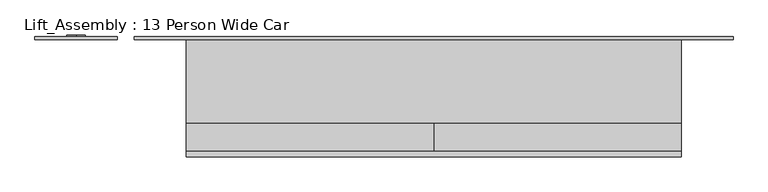
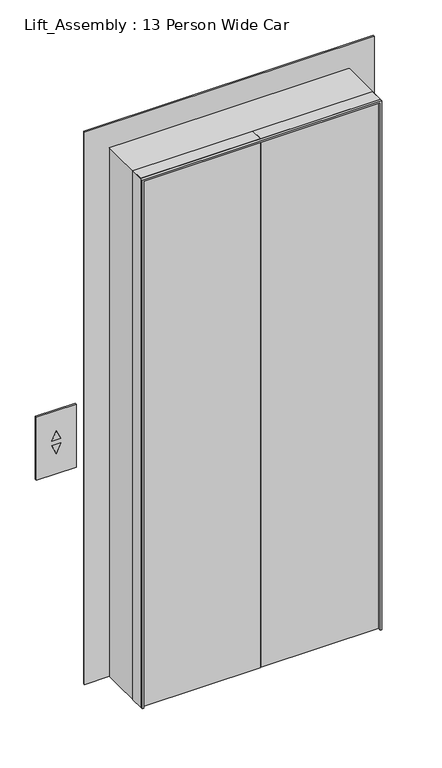
"""IFC4 building model written with IfcOpenShell, lengths in millimetres: proxy geometry, Lift_Assembly : 13 Person Wide Car."""

from ifc_helpers import new_model, si_unit, frame, origin, origin_with_axes, place, context, project, spatial, polyline, outline, extrude, faceted_brep, source, transform, mapped, element, save


def lift_assembly_13_person_wide_car_ee12aecb(model_context):
    return source(origin(), model_context, "Body", "SolidModel", [
        extrude(outline(polyline([(200.0, -126.2), (-249.0, -126.2), (-249.0, -76.2), (200.0, -76.2), (200.0, -126.2)])), origin_with_axes(), (0.0, 0.0, 1.0), 2100.0),
        extrude(outline(polyline([(-250.0, -126.2), (-700.0, -126.2), (-700.0, -76.2), (-250.0, -76.2), (-250.0, -126.2)])), origin_with_axes(), (0.0, 0.0, 1.0), 2100.0),
        extrude(outline(polyline([(1008.7476885, -883.0952695), (1045.0, -900.0), (1008.7476885, -916.9047305), (1008.7476885, -883.0952695)])), frame((0.0, 76.2, 0.0), z_axis=(0.0, 1.0, 0.0), x_axis=(0.0, 0.0, 1.0)), (0.0, 0.0, 1.0), 9.0),
        extrude(outline(polyline([(991.2523115, -883.0952695), (991.2523115, -916.9047305), (955.0, -900.0), (991.2523115, -883.0952695)])), frame((0.0, 76.2, 0.0), z_axis=(0.0, 1.0, 0.0), x_axis=(0.0, 0.0, 1.0)), (0.0, 0.0, 1.0), 9.0),
        faceted_brep([(294.0, 82.2, 0.0), (294.0, 76.2, 0.0), (200.0, 76.2, 0.0), (200.0, -136.8, 0.0), (194.0, -136.8, 0.0), (194.0, 82.2, 0.0), (294.0, 82.2, 2194.0), (294.0, 76.2, 2194.0), (-794.0, 76.2, 2194.0), (-794.0, 76.2, 0.0), (-700.0, 76.2, 0.0), (-700.0, 76.2, 2100.0), (200.0, 76.2, 2100.0), (200.0, -136.8, 2100.0), (-700.0, -136.8, 2100.0), (-700.0, -136.8, 0.0), (-694.0, -136.8, 0.0), (-694.0, -136.8, 2094.0), (194.0, -136.8, 2094.0), (194.0, 82.2, 2094.0), (-694.0, 82.2, 2094.0), (-694.0, 82.2, 0.0), (-794.0, 82.2, 0.0), (-794.0, 82.2, 2194.0)], [[[0, 1, 2, 3, 4, 5]], [[1, 0, 6, 7]], [[2, 1, 7, 8, 9, 10, 11, 12]], [[3, 2, 12, 13]], [[4, 3, 13, 14, 15, 16, 17, 18]], [[5, 4, 18, 19]], [[0, 5, 19, 20, 21, 22, 23, 6]], [[7, 6, 23, 8]], [[13, 12, 11, 14]], [[19, 18, 17, 20]], [[22, 21, 16, 15, 10, 9]], [[8, 23, 22, 9]], [[14, 11, 10, 15]], [[20, 17, 16, 21]]]),
        extrude(outline(polyline([(875.0, -975.0), (875.0, -825.0), (1125.0, -825.0), (1125.0, -975.0), (875.0, -975.0)]), holes=[polyline([(1008.7476885, -883.0952695), (1008.7476885, -916.9047305), (1045.0, -900.0), (1008.7476885, -883.0952695)]), polyline([(991.2523115, -883.0952695), (955.0, -900.0), (991.2523115, -916.9047305), (991.2523115, -883.0952695)])]), frame((0.0, 76.2, 0.0), z_axis=(0.0, 1.0, 0.0), x_axis=(0.0, 0.0, 1.0)), (0.0, 0.0, 1.0), 6.0),
    ])


if __name__ == "__main__":
    model = new_model("IFC4")
    model_context = context("Model", 3, world=origin())
    ifc_project = project(units=[si_unit("LENGTHUNIT", "METRE", prefix="MILLI")], contexts=[model_context])
    site = spatial("IfcSite", under=ifc_project)
    building = spatial("IfcBuilding", under=site)
    placement = place(None, origin())
    lift_assembly_13_person_wide_car_shape = lift_assembly_13_person_wide_car_ee12aecb(model_context)
    element("IfcBuildingElementProxy", 1, Name="Lift_Assembly : 13 Person Wide Car", ObjectType="Lift_Assembly : 13 Person Wide Car", at=placement, inside=building, context=model_context, shape_type="MappedRepresentation", body=[
        mapped(lift_assembly_13_person_wide_car_shape, transform((0.0, 0.0, 0.0), x_axis=(1.0, 0.0, 0.0), y_axis=(0.0, 1.0, 0.0), z_axis=(0.0, 0.0, 1.0))),
    ])
    save(model, "model.ifc")

# Revit data of these elements
# Type "Lift_Assembly : 13 Person Wide Car"
#   Keynote = "X"
#   Hoistway Width = 2400 mm
#   Hoistway Depth = 1800 mm
#   Height = 2100 mm
#   Frame Width = 75 mm
#   Percentage Opened (Plan) = 0 mm
#   Door Width = 900 mm
#   Door Trim Width = 100 mm
#   Door Thickness = 50 mm
#   Car Width = 1600 mm
#   Car Thickness = 25 mm
#   Car Front Offset = 250 mm
#   Car Depth = 1400 mm
#   Call Point Z Offset = 1000 mm
#   Call Point X Offset = 200 mm
#   Call Point Panel Width = 150 mm
#   Call Point Panel Depth = 250 mm
#   Vis - Hoistway Location Lines = yes
#   Vis - Door Trim = yes
#   Vis - Call Point = yes
#   Material Trim = Metal - Stainless Steel
#   Material Doors = Metal - Aluminium
#   Wall Closure = (empty or 0)
#   Default Elevation = 0
# Element 1 (IfcBuildingElementProxy, "Lift_Assembly : 13 Person Wide Car")
#   Materials on its faces: "Metal - Stainless Steel", "Metal - Aluminium"
# Materials
#   "Metal - Stainless Steel": class "Metal", colour RGB 247 247 247, transparency 0
#   "Metal - Aluminium": class "Metal", colour RGB 247 247 247, transparency 0
